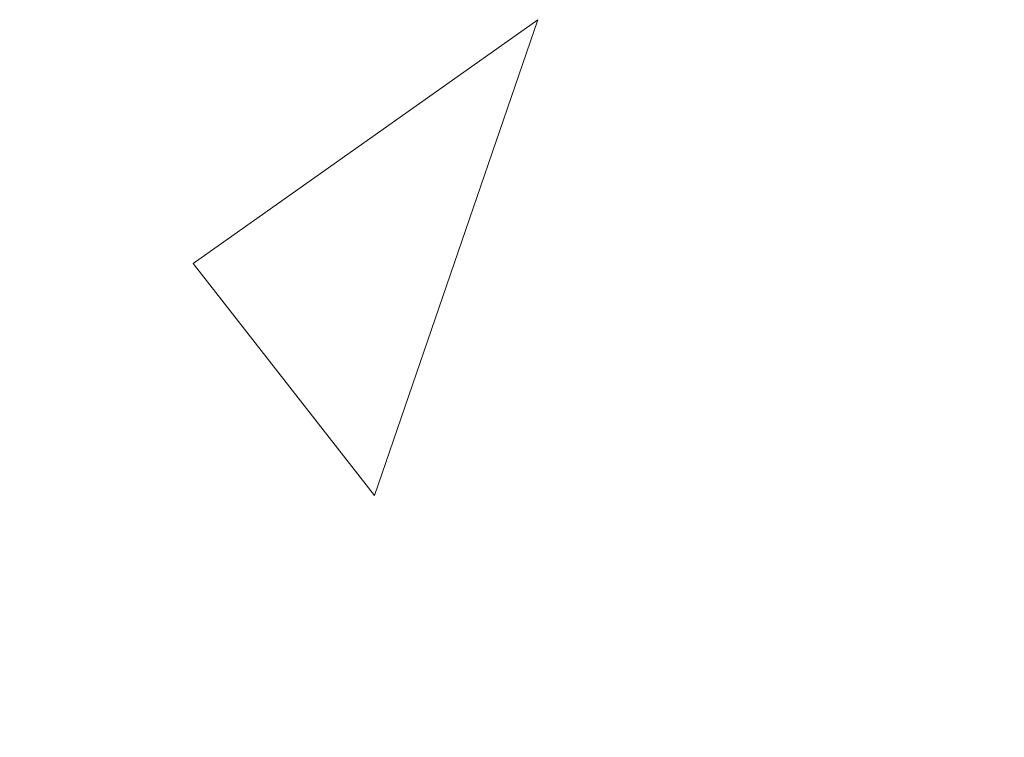
# Model space of a CAD drawing. Units: inches. Extents: x 459864 to 460310, y 324185 to 324787.
# Tile 8 of 112: x 460070.4681 to 460071.2168, y 324239.6755 to 324240.221. Entities that reach past the tile are written whole.
import ezdxf

# ---------------------------------------------------------------- set-up
doc = ezdxf.new("R2010")
doc.units = ezdxf.units.IN
doc.layers.add('A-ANNO-DIMS', color=2, linetype='Continuous', lineweight=18)
doc.layers.add('L-HRDS', color=9, linetype='Continuous', lineweight=18)
doc.styles.get("Standard").update_dxf_attribs({"font": 'arial.ttf'})
doc.dimstyles.new('ISO-25', dxfattribs={"dimtxt": 6, "dimasz": 2.5, "dimexe": 1.25, "dimexo": 0.625, "dimtad": 1, "dimdec": 1, "dimlunit": 3, "dimtxsty": 'Standard', "dimcen": 2.5, "dimadec": 0, "dimazin": 0, "dimtfac": 1, "dimtdec": 1, "dimtmove": 0, "dimatfit": 3, "dimfxl": 1, "dimarcsym": 0})

# ---------------------------------------------------------------- blocks, each defined once
blk = doc.blocks.new('Stepping Stone - hexagonal')
for p, q in [((0.7041, 8.5646), (0.2671, 8.2556)), ((0.4971, 7.9616), (0.7041, 8.5646)), ((0.2671, 8.2556), (0.4971, 7.9616))]:
    blk.add_line(p, q)
blk = doc.blocks.new('*D36')
at = {"layer": 'A-ANNO-DIMS', "color": 0, "lineweight": -2, "transparency": 16777216}
for p, q in [((460063.86135, 324228.48284), (460063.86135, 324226.05568)), ((460075.87575, 324228.48284), (460075.87575, 324226.05568)), ((460066.36135, 324227.30568), (460073.37575, 324227.30568)), ((460075.87575, 324227.30568), (460126.02138, 324227.30568))]:
    blk.add_line(p, q, dxfattribs=at)
at = {"layer": 'A-ANNO-DIMS', "color": 0, "transparency": 16777216}
for points in [[(460066.36135, 324227.72234), (460066.36135, 324226.88901), (460063.86135, 324227.30568)], [(460073.37575, 324227.72234), (460073.37575, 324226.88901), (460075.87575, 324227.30568)]]:
    blk.add_solid(points, dxfattribs=at)
at = {"layer": 'Defpoints', "color": 0, "transparency": 16777216}
for p in [(460063.86135, 324229.10784), (460075.87575, 324229.10784), (460075.87575, 324227.30568)]:
    blk.add_point(p, dxfattribs=at)
at = {"layer": 'A-ANNO-DIMS', "color": 0, "transparency": 16777216, "insert": (460102.19857, 324230.99411), "char_height": 6, "attachment_point": 5}
blk.add_mtext('PAVER 1\'-0"', dxfattribs=at)

msp = doc.modelspace()

# ---------------------------------------------------------------- block references
at = {"layer": 'L-HRDS', "xscale": 0.6, "yscale": 0.6}
msp.add_blockref('Stepping Stone - hexagonal', (460070.43968, 324235.08229), dxfattribs=at)

# ---------------------------------------------------------------- dimensions: what is measured, and where the dimension line sits
at = {"layer": 'A-ANNO-DIMS'}
dim = msp.add_linear_dim(base=(460075.87575, 324227.30568), p1=(460063.86135, 324229.10784), p2=(460075.87575, 324229.10784), text='PAVER <>', dimstyle='ISO-25', override={"dimdec": 1, "dimlfac": 1, "dimrnd": 0, "dimzin": 1, "dimdsep": 46, "dimlunit": 4, "dimfrac": 2}, dxfattribs=at)
dim.commit()
dim.dimension.update_dxf_attribs({"geometry": '*D36', "text_midpoint": (460102.19857, 324230.99411)})

doc.saveas('drawing.dxf')
